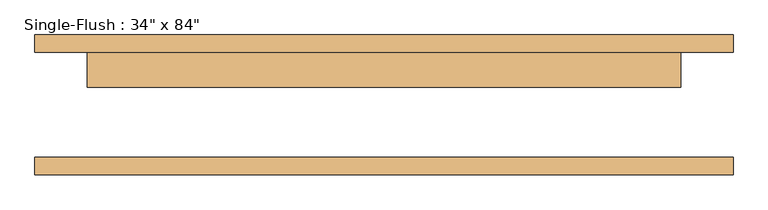
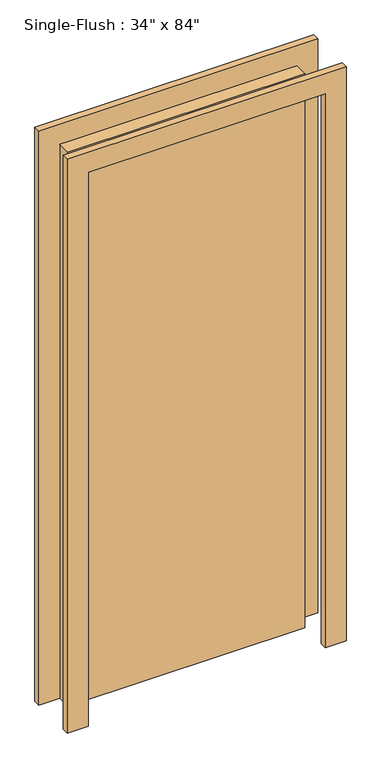
"""IFC4 building model written with IfcOpenShell, lengths in millimetres: door geometry."""

from ifc_helpers import new_model, si_unit, frame, origin, origin_with_axes, place, context, project, spatial, polyline, outline, extrude, source, transform, mapped, element, save


def door_b6e9fca3(model_context):
    return source(origin(), model_context, "Body", "SweptSolid", [
        extrude(outline(polyline([(2209.8, -508.0), (0.0, -508.0), (0.0, -431.8), (2133.6, -431.8), (2133.6, 431.8), (0.0, 431.8), (0.0, 508.0), (2209.8, 508.0), (2209.8, -508.0)])), frame((0.0, 76.2, 0.0), z_axis=(0.0, 1.0, 0.0), x_axis=(0.0, 0.0, 1.0)), (0.0, 0.0, 1.0), 25.4),
        extrude(outline(polyline([(2209.8, 508.0), (2209.8, -508.0), (0.0, -508.0), (0.0, -431.8), (2133.6, -431.8), (2133.6, 431.8), (0.0, 431.8), (0.0, 508.0), (2209.8, 508.0)])), frame((0.0, -101.6, 0.0), z_axis=(0.0, 1.0, 0.0), x_axis=(0.0, 0.0, 1.0)), (0.0, 0.0, 1.0), 25.4),
        extrude(outline(polyline([(431.8, 25.4), (-431.8, 25.4), (-431.8, 76.2), (431.8, 76.2), (431.8, 25.4)])), origin_with_axes(), (0.0, 0.0, 1.0), 2133.6),
    ])


if __name__ == "__main__":
    model = new_model("IFC4")
    model_context = context("Model", 3, world=origin())
    ifc_project = project(units=[si_unit("LENGTHUNIT", "METRE", prefix="MILLI")], contexts=[model_context])
    site = spatial("IfcSite", under=ifc_project)
    building = spatial("IfcBuilding", under=site)
    placement = place(None, origin())
    door_shape = door_b6e9fca3(model_context)
    element("IfcDoor", 1, ObjectType="Single-Flush : 34\" x 84\"", at=placement, inside=building, context=model_context, shape_type="MappedRepresentation", body=[
        mapped(door_shape, transform((0.0, 0.0, 0.0), x_axis=(1.0, 0.0, 0.0), y_axis=(0.0, 1.0, 0.0), z_axis=(0.0, 0.0, 1.0))),
    ])
    save(model, "model.ifc")

# Revit data of these elements
# Type "Single-Flush : 34\" x 84\""
#   Type Mark = "2"
#   Construction Type Id = "MDOOR"
#   Assembly Code = "C1020"
#   Analytic Construction = "Metal"
#   Thickness = 0' - 2"
#   Heat Transfer Coefficient (U) = 0.651978 BTU/(h·ft²·°F)
#   Height = 7' - 0"
#   Trim Projection Ext = 0' - 1"
#   Trim Projection Int = 0' - 1"
#   Trim Width = 0' - 3"
#   Width = 2' - 10"
#   Define Thermal Properties by = 1
#   Define Thermal Properties by = 1
#   Door Material = Door - Panel
#   Frame Material = Door - Frame
#   Visual Light Transmittance = 0
#   Solar Heat Gain Coefficient = 0
#   Function = (empty or 0)
#   Wall Closure = (empty or 0)
# Element 1 (IfcDoor, "Single-Flush : 34\" x 84\"")
#   Materials on its faces: "Door - Frame", "Door - Panel"
# Materials
#   "Door - Panel": class "Wood", colour RGB 210 159 95, transparency 0, Cost = 0
#   "Door - Frame": colour RGB 118 70 51, transparency 0, Cost = 0
